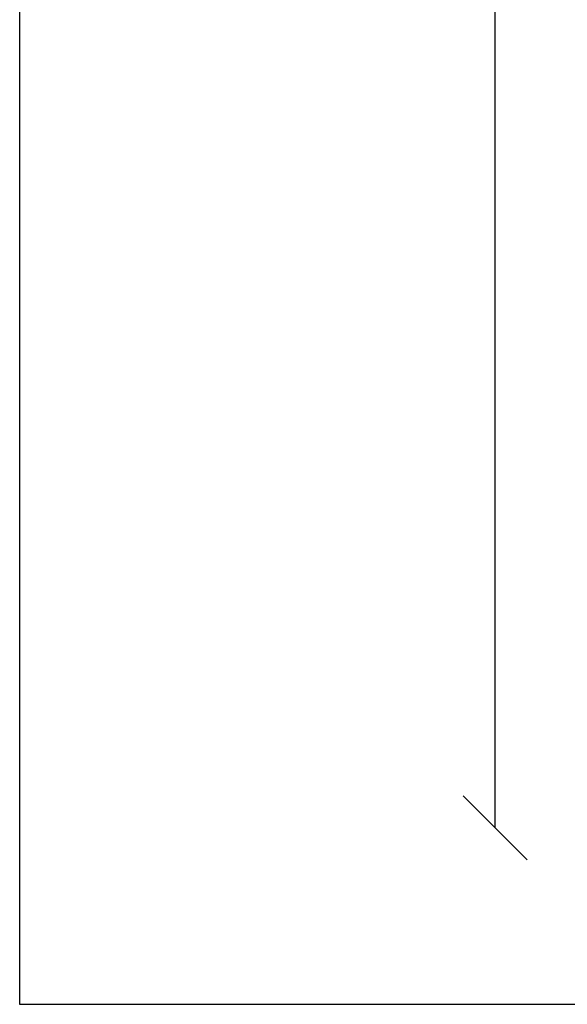
# Model space of a CAD drawing. Units: inches. Extents: x 311 to 815, y -527 to 136.
# Tile 1 of 21: x 311 to 388, y -507 to -368. Entities that reach past the tile are written whole.
import ezdxf

# ---------------------------------------------------------------- set-up
doc = ezdxf.new("R2010")
doc.units = ezdxf.units.IN
doc.header["$MEASUREMENT"] = 0
doc.layers.add('A-ANNO-DIMS', color=1, linetype='Continuous', lineweight=18)
doc.layers.add('A-ANNO-TTLB', color=1, linetype='Continuous', lineweight=25)
doc.styles.get("Standard").update_dxf_attribs({"font": 'arial.ttf'})
doc.dimstyles.get("Standard").update_dxf_attribs({"dimtxt": 0.18, "dimasz": 0.18, "dimexe": 0.18, "dimexo": 0.0625, "dimgap": 0.09, "dimtad": 0, "dimtih": 1, "dimtoh": 1, "dimdec": 1, "dimzin": 0, "dimdsep": 46, "dimlunit": 4, "dimtxsty": 'Standard', "dimcen": 0.09, "dimadec": 0, "dimazin": 0, "dimtfac": 1, "dimtdec": 1, "dimtofl": 0, "dimtmove": 0, "dimatfit": 3, "dimfxl": 1, "dimtolj": 1, "dimtzin": 0, "dimarcsym": 0})

# ---------------------------------------------------------------- blocks, each defined once
blk = doc.blocks.new('_ArchTick')
at = {"color": 0, "linetype": 'ByBlock', "const_width": 0.15}
blk.add_lwpolyline([(-0.5, -0.5), (0.5, 0.5)], dxfattribs=at)
blk = doc.blocks.new('_Oblique')
at = {"color": 0, "linetype": 'ByBlock', "lineweight": -2}
blk.add_line((-0.5, -0.5), (0.5, 0.5), dxfattribs=at)
blk = doc.blocks.new('*D3')
at = {"layer": 'A-ANNO-DIMS', "color": 0, "lineweight": -2, "transparency": 16777216}
for p, q in [((377.54, 21.87), (377.54, -221.61)), ((377.54, -482.13), (377.54, -238.65))]:
    blk.add_line(p, q, dxfattribs=at)
at = {"layer": 'Defpoints', "color": 0, "transparency": 16777216}
for p in [(410.32, 21.87), (377.54, -482.13), (410.32, -482.13)]:
    blk.add_point(p, dxfattribs=at)
at = {"layer": 'A-ANNO-DIMS', "color": 0, "lineweight": -2, "transparency": 16777216, "xscale": 9, "yscale": 9, "zscale": 9}
for name, p, rotation in [('_ArchTick', (377.54, 21.87), 90), ('_Oblique', (377.54, -482.13), 270)]:
    blk.add_blockref(name, p, dxfattribs=dict(at, rotation=rotation))
at = {"layer": 'A-ANNO-DIMS', "color": 0, "transparency": 16777216, "insert": (377.54, -230.13), "char_height": 9, "attachment_point": 5}
blk.add_mtext("\\A1;42'", dxfattribs=at)

msp = doc.modelspace()

# ---------------------------------------------------------------- linework, layer by layer
at = {"layer": 'A-ANNO-TTLB'}
msp.add_lwpolyline([(310.67, 136.01), (815.43, 136.01), (815.43, -506.97), (310.67, -506.97)], close=True, dxfattribs=at)

# ---------------------------------------------------------------- dimensions: what is measured, and where the dimension line sits
at = {"layer": 'A-ANNO-DIMS'}
dim = msp.add_linear_dim(base=(377.54, -482.13), p1=(410.32, 21.87), p2=(410.32, -482.13), angle=90, dimstyle='Standard', override={"dimtxt": 9, "dimasz": 9, "dimgap": 4, "dimblk1": 'ArchTick', "dimblk2": 'Oblique', "dimsah": 1, "dimse1": 1, "dimse2": 1, "dimclrd": 0, "dimclre": 0, "dimclrt": 0}, dxfattribs=at)
dim.commit()
dim.dimension.update_dxf_attribs({"geometry": '*D3', "text_midpoint": (377.54, -230.13)})

doc.saveas('drawing.dxf')
